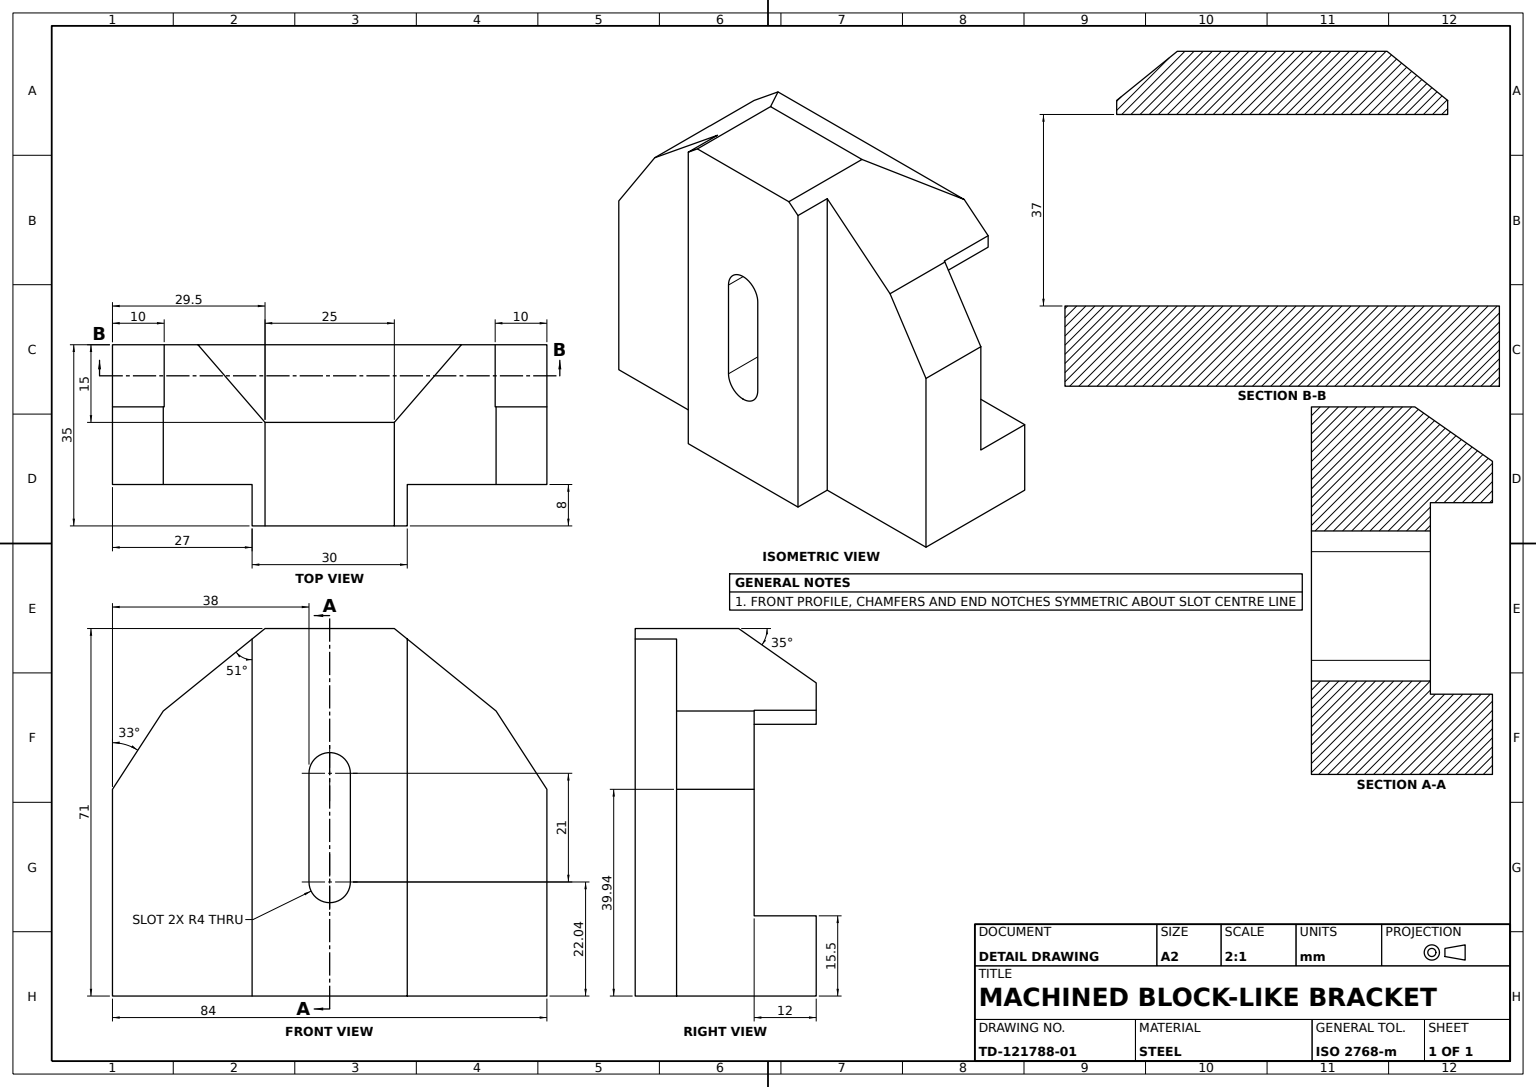
SolidWorks part; units mm, degrees
material "Plain Carbon Steel"
ref_plane "Front Plane" through (0, 0, 0) normal (0, 0, 1) x (1, 0, 0)
ref_plane "Top Plane" through (0, 0, 0) normal (0, 1, 0) x (1, 0, 0)
ref_plane "Right Plane" through (0, 0, 0) normal (1, 0, 0) x (0, 0, -1)
sketch "Block Profile Sketch" plane through (0, 0, 0) normal (0, 0, 1) x (1, 0, 0)
  line L0 (0, 0) -> (27, 0)
  line L1 (27, 0) -> (27, 71)
  line L2 (27, 71) -> (15, 71)
  line L3 (0, 60.4969) -> (0, 52.4969)
  line L4 (0, 52.4969) -> (12, 52.4969)
  line L5 (12, 52.4969) -> (12, 15.4969)
  line L6 (12, 15.4969) -> (0, 15.4969)
  line L7 (0, 15.4969) -> (0, 0)
  line L8 (15, 71) -> (0, 60.4969)
  point P5 (0, 71)
  dimension "D1" = 71
  dimension "D2" = 37
  dimension "D3" = 27
  dimension "D4" = 15
  dimension "D5" = 35
  dimension "D6" = 8
  dimension "D7" = 12
extrude "Base Block 84mm" add sketch "Block Profile Sketch" along normal blind 84
sketch "Back Channel Sketch" plane through (0, 15.4969, 0) normal (0, 1, 0) x (1, 0, 0)
  line L0 (12, -84) -> (12, 0) construction
  line L1 (0, -84) -> (12, -84)
  line L2 (0, -84) -> (0, -74)
  line L3 (0, -74) -> (12, -74)
  line L4 (12, -84) -> (12, -74)
  line L6 (0, 0) -> (12, 0)
  line L7 (0, 0) -> (0, -10)
  line L8 (0, -10) -> (12, -10)
  line L9 (12, 0) -> (12, -10)
  dimension "D1" = 10
  dimension "D2" = 10
extrude "Back Channel Cut" cut sketch "Back Channel Sketch" along normal blind 84
ref_plane "Front Pad Plane" through (0, 0, 42) normal (0, 0, 1) x (1, 0, 0)
sketch "Front Pad Sketch" plane through (0, 0, 42) normal (0, 0, 1) x (1, 0, 0)
  line L0 (27, 0) -> (27, 71) construction
  line L1 (27, 71) -> (35, 71)
  line L2 (27, 71) -> (27, 0)
  line L3 (27, 0) -> (35, 0)
  line L4 (35, 71) -> (35, 0)
  line L5 (0, 0) -> (27, 0) construction
  line L6 (27, 71) -> (15, 71) construction
  dimension "D1" = 8
extrude "Front Pad 8mm" add sketch "Front Pad Sketch" along normal mid plane 30
sketch "Top Chamfer Sketch" plane through (27, 0, 0) normal (1, 0, 0) x (0, 0, -1)
  line L0 (-54.5, 71) -> (-74.1756, 55.067)
  line L1 (-42, 71) -> (-42, -9.7878) construction
  line L2 (-42, 14.85) -> (-42, -14.85) construction
  line L3 (-27, 71) -> (-27, 0) construction
  line L4 (-84, 0) -> (-84, 71) construction
  line L6 (-84, 39.9388) -> (-74.1756, 55.067)
  line L7 (-29.5, 71) -> (-9.8244, 55.067)
  line L8 (0, 39.9388) -> (-9.8244, 55.067)
  line L11 (0, 0) -> (0, 71) construction
  line L12 (-27, 71) -> (0, 71) construction
  line L13 (-84, 71) -> (-57, 71) construction
  line L14 (0, 39.9388) -> (0, 71)
  line L15 (-29.5, 71) -> (0, 71)
  line L16 (-84, 39.9388) -> (-84, 71)
  line L17 (-84, 71) -> (-54.5, 71)
  dimension "D1" = 51
  dimension "D2" = 12.5
  dimension "D3" = 12.5
  dimension "D4" = 33
  dimension "D5" = 17.1756
extrude "Top Chamfer Cut" cut sketch "Top Chamfer Sketch" against normal mid plane 85
sketch "Slot Sketch" plane through (12, 0, 0) normal (-1, 0, 0) x (0, 0, 1)
  line L0 (42, 43.0356) -> (42, 22.0356) construction
  line L1 (46, 43.0356) -> (46, 22.0356)
  line L2 (38, 43.0356) -> (38, 22.0356)
  line L3 (0, 15.4969) -> (0, 0) construction
  line L4 (84, 15.4969) -> (0, 15.4969) construction
  arc A0 (46, 43.0356) -> (38, 43.0356) centre (42, 43.0356) ccw
  arc A1 (38, 22.0356) -> (46, 22.0356) centre (42, 22.0356) ccw
  point P2 (42, 32.5356)
  dimension "D1" = 4
  dimension "D2" = 42
  dimension "D3" = 21
  dimension "D4" = 6.5387
extrude "Slot Cut" cut sketch "Slot Sketch" against normal blind 75
